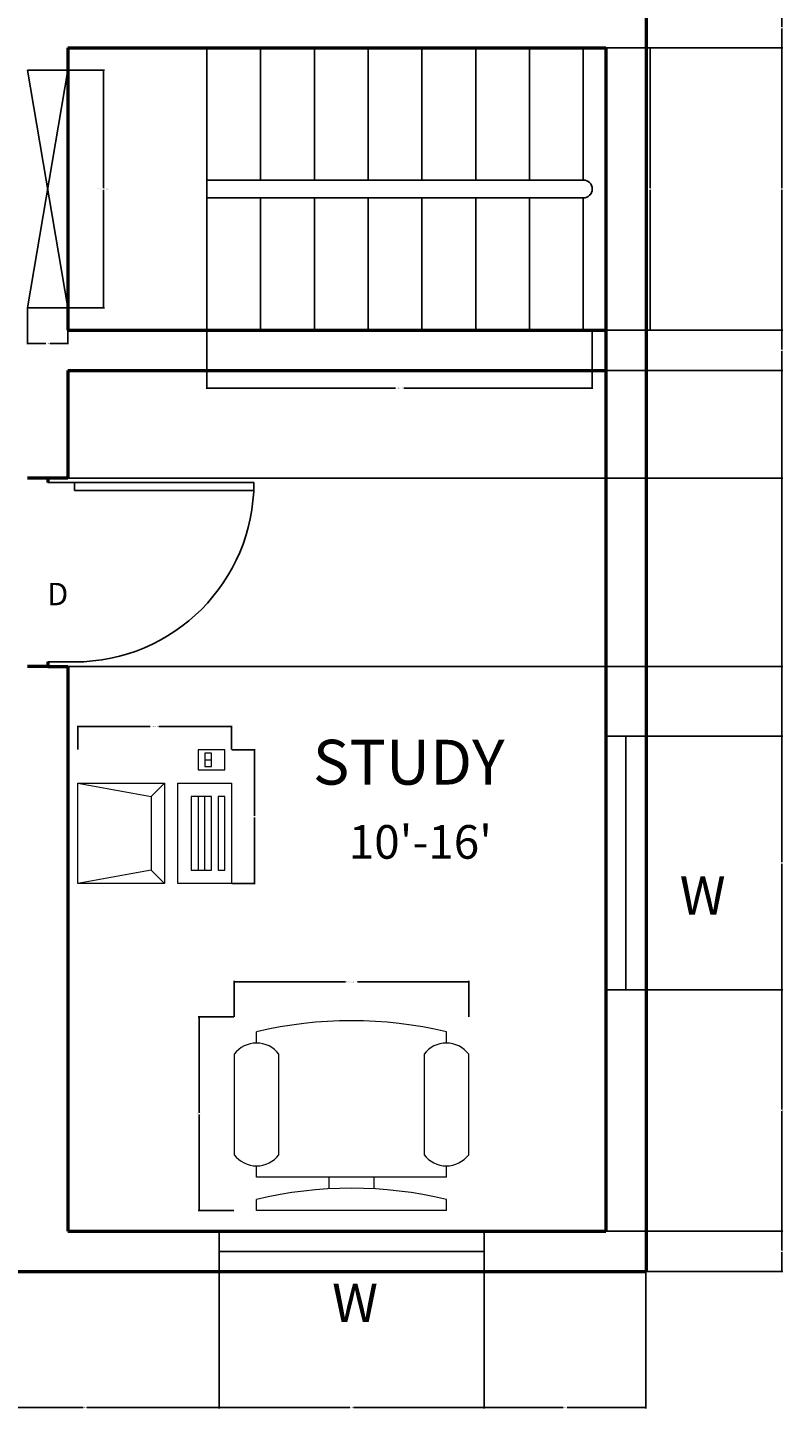
# Model space of a CAD drawing. Units: inches. Extents: x 2164 to 3752, y 2015 to 2629.
# Tile 6 of 8: x 3583 to 3752, y 2015 to 2323. Entities that reach past the tile are written whole.
import ezdxf
from ezdxf.enums import TextEntityAlignment as Align

# ---------------------------------------------------------------- set-up
doc = ezdxf.new("R2010")
doc.units = ezdxf.units.IN
for name, color, linetype, lineweight in [('A-ANNO-DIMS', 2, 'Continuous', 18), ('A-ANNO-TEXT', 7, 'Continuous', 25), ('A-AREA-IDEN', 3, 'Continuous', 25), ('A-DOOR', 3, 'Continuous', 25), ('A-FLOR-STRS', 2, 'Continuous', 25), ('A-FURN', 8, 'Continuous', 18), ('A-GLAZ', 4, 'Continuous', 25), ('A-WALL', 7, 'Continuous', 50)]:
    doc.layers.add(name, color=color, linetype=linetype, lineweight=lineweight)
doc.styles.get("Standard").update_dxf_attribs({"font": 'arial.ttf'})
doc.dimstyles.get("Standard").update_dxf_attribs({"dimtxt": 0.18, "dimasz": 0.18, "dimexe": 0.18, "dimexo": 0.0625, "dimgap": 0.09, "dimtad": 0, "dimtih": 1, "dimtoh": 1, "dimdec": 4, "dimzin": 0, "dimdsep": 46, "dimtxsty": 'Standard', "dimcen": 0.09, "dimadec": 0, "dimazin": 0, "dimtfac": 1, "dimtdec": 4, "dimtofl": 0, "dimtmove": 0, "dimatfit": 3, "dimfxl": 1, "dimtolj": 1, "dimtzin": 0, "dimarcsym": 0})

# ---------------------------------------------------------------- blocks, each defined once
blk = doc.blocks.new('*U7')
for p, q in [((0, 0), (0, -6)), ((40, 0), (40, -6))]:
    blk.add_line(p, q)
blk.add_lwpolyline([(0, 0), (0, 40), (1.75, 40), (1.75, 0)], close=True)
blk.add_arc((0, 0), 40, 0, 90)
blk = doc.blocks.new('Chair - Desk')
for p, q in [((-8.5, 0), (-8.5, -1)), ((-8.5, 0), (8.5, 0)), ((8.5, 0), (8.5, -1)), ((-2, -3), (-2, -1.9355)), ((2, -1.9576), (2, -3)), ((-8.5, -3), (-8.5, -4)), ((-8.5, -3), (8.5, -3)), ((8.5, -3), (8.5, -4)), ((-10.5, -5), (-10.5, -14)), ((-6.5, -14), (-6.5, -5)), ((6.5, -5), (6.5, -14)), ((10.5, -14), (10.5, -5)), ((-8.5, -15), (-8.5, -16)), ((8.5, -15), (8.5, -16))]:
    blk.add_line(p, q)
for centre, radius, start, end in [((0, 34.625), 36.625, 256.5803, 283.4197), ((-8.5, -6.5), 2.5, 36.8699, 143.1301), ((8.5, -6.5), 2.5, 36.8699, 143.1301), ((-8.5, -12.5), 2.5, 216.8699, 323.1301), ((8.5, -12.5), 2.5, 216.8699, 323.1301), ((0, 19.625), 36.625, 256.5803, 283.4197)]:
    blk.add_arc(centre, radius, start, end)
blk = doc.blocks.new('Computer Terminal')
for p, q in [((-10, 11.5), (5, 11.5)), ((-8, 0.5), (-10, 11.5)), ((-10, -1.5), (-10, 11.5)), ((5, 11.5), (3, 0.5)), ((5, 11.5), (5, -1.5)), ((-10, -1.5), (-8, 0.5)), ((3, 0.5), (-8, 0.5)), ((3, 0.5), (5, -1.5)), ((5, -1.5), (-10, -1.5)), ((-10, -11.5), (-10, -3.5)), ((-10, -3.5), (5, -3.5)), ((5, -3.5), (5, -11.5)), ((-8, -5.5), (-8, -8.5)), ((3, -5.5), (-8, -5.5)), ((3, -8.5), (3, -5.5)), ((3, -6.5), (-8, -6.5)), ((-8, -7.5), (3, -7.5)), ((10, -6.5), (7, -6.5)), ((7, -6.5), (7, -10.5)), ((9.5, -7.5), (7.5, -7.5)), ((7.5, -7.5), (7.5, -8.5)), ((8.5, -7.5), (8.5, -8.5)), ((9.5, -8.5), (9.5, -7.5)), ((10, -10.5), (10, -6.5)), ((-8, -8.5), (3, -8.5)), ((-8, -9.5), (-8, -10.5)), ((3, -9.5), (-8, -9.5)), ((3, -10.5), (3, -9.5)), ((7.5, -8.5), (9.5, -8.5)), ((5, -11.5), (-10, -11.5)), ((-8, -10.5), (3, -10.5)), ((7, -10.5), (10, -10.5))]:
    blk.add_line(p, q)
blk = doc.blocks.new('STAIR-HANDRAIL')
for p, q in [((84, 63), (84, 33.5)), ((0, 33.5), (84, 33.5)), ((0, 29.5), (84, 29.5)), ((84, 29.5), (84, 0))]:
    blk.add_line(p, q)
blk.add_arc((84, 31.5), 2, 270, 90)
blk = doc.blocks.new('VENT-OPENING')
for p, q in [((9, 53), (0, 53)), ((9, 53), (0, 0)), ((9, 0), (0, 53)), ((9, 0), (0, 0))]:
    blk.add_line(p, q)
blk = doc.blocks.new('*D25')
at = {"layer": 'A-ANNO-DIMS', "color": 0, "lineweight": -2, "transparency": 16777216}
for p, q in [((3629.5, 2102.57), (3629.5, 2110.54)), ((3629.68, 2110.36), (3654.34, 2110.36)), ((3681.65, 2110.36), (3656.99, 2110.36)), ((3681.83, 2102.57), (3681.83, 2110.54))]:
    blk.add_line(p, q, dxfattribs=at)
at = {"layer": 'A-ANNO-DIMS', "color": 0, "transparency": 16777216}
for points in [[(3629.68, 2110.39), (3629.68, 2110.33), (3629.5, 2110.36)], [(3681.65, 2110.39), (3681.65, 2110.33), (3681.83, 2110.36)]]:
    blk.add_solid(points, dxfattribs=at)
at = {"layer": 'Defpoints', "color": 0, "transparency": 16777216}
for p in [(3629.5, 2110.36), (3629.5, 2102.51), (3681.83, 2102.51)]:
    blk.add_point(p, dxfattribs=at)
at = {"layer": 'A-ANNO-DIMS', "color": 0, "transparency": 16777216, "insert": (3655.66, 2110.36), "char_height": 0.18, "attachment_point": 5}
blk.add_mtext('\\A1;DESK CHAIR 52 TYP.', dxfattribs=at)
blk = doc.blocks.new('*D26')
at = {"layer": 'A-ANNO-DIMS', "color": 0, "lineweight": -2, "transparency": 16777216}
for p, q in [((3629.44, 2102.51), (3621.47, 2102.51)), ((3621.65, 2102.33), (3621.65, 2081.1)), ((3621.65, 2059.5), (3621.65, 2080.73)), ((3629.44, 2059.32), (3621.47, 2059.32))]:
    blk.add_line(p, q, dxfattribs=at)
at = {"layer": 'A-ANNO-DIMS', "color": 0, "transparency": 16777216}
for points in [[(3621.62, 2102.33), (3621.68, 2102.33), (3621.65, 2102.51)], [(3621.62, 2059.5), (3621.68, 2059.5), (3621.65, 2059.32)]]:
    blk.add_solid(points, dxfattribs=at)
at = {"layer": 'Defpoints', "color": 0, "transparency": 16777216}
for p in [(3629.5, 2102.51), (3621.65, 2059.32), (3629.5, 2059.32)]:
    blk.add_point(p, dxfattribs=at)
at = {"layer": 'A-ANNO-DIMS', "color": 0, "transparency": 16777216, "insert": (3621.65, 2080.92), "char_height": 0.18, "attachment_point": 5}
blk.add_mtext('\\A1;43 TYP.', dxfattribs=at)
blk = doc.blocks.new('*D31')
at = {"layer": 'A-ANNO-DIMS', "color": 0, "lineweight": -2, "transparency": 16777216}
for p, q in [((3623.39, 2255.65), (3623.39, 2242.64)), ((3709.39, 2255.65), (3709.39, 2242.64)), ((3623.57, 2242.82), (3665.46, 2242.82)), ((3709.21, 2242.82), (3667.33, 2242.82))]:
    blk.add_line(p, q, dxfattribs=at)
at = {"layer": 'A-ANNO-DIMS', "color": 0, "transparency": 16777216}
for points in [[(3623.57, 2242.85), (3623.57, 2242.79), (3623.39, 2242.82)], [(3709.21, 2242.85), (3709.21, 2242.79), (3709.39, 2242.82)]]:
    blk.add_solid(points, dxfattribs=at)
at = {"layer": 'Defpoints', "color": 0, "transparency": 16777216}
for p in [(3623.39, 2255.72), (3709.39, 2255.72), (3709.39, 2242.82)]:
    blk.add_point(p, dxfattribs=at)
at = {"layer": 'A-ANNO-DIMS', "color": 0, "transparency": 16777216, "insert": (3666.39, 2242.82), "char_height": 0.18, "attachment_point": 5}
blk.add_mtext('\\A1;STAIR 86 TYP.', dxfattribs=at)
blk = doc.blocks.new('*D32')
at = {"layer": 'A-ANNO-DIMS', "color": 0, "lineweight": -2, "transparency": 16777216}
for p, q in [((3709.46, 2318.72), (3722.47, 2318.72)), ((3722.29, 2318.54), (3722.29, 2287.4)), ((3722.29, 2255.9), (3722.29, 2287.04)), ((3709.46, 2255.72), (3722.47, 2255.72))]:
    blk.add_line(p, q, dxfattribs=at)
at = {"layer": 'A-ANNO-DIMS', "color": 0, "transparency": 16777216}
for points in [[(3722.26, 2318.54), (3722.32, 2318.54), (3722.29, 2318.72)], [(3722.26, 2255.9), (3722.32, 2255.9), (3722.29, 2255.72)]]:
    blk.add_solid(points, dxfattribs=at)
at = {"layer": 'Defpoints', "color": 0, "transparency": 16777216}
for p in [(3709.39, 2318.72), (3722.29, 2318.72), (3709.39, 2255.72)]:
    blk.add_point(p, dxfattribs=at)
at = {"layer": 'A-ANNO-DIMS', "color": 0, "transparency": 16777216, "insert": (3722.29, 2287.22), "char_height": 0.18, "attachment_point": 5}
blk.add_mtext('\\A1;63 TYP.', dxfattribs=at)
blk = doc.blocks.new('*D33')
at = {"layer": 'A-ANNO-DIMS', "color": 0, "lineweight": -2, "transparency": 16777216}
for p, q in [((3592.46, 2313.72), (3600.52, 2313.72)), ((3600.34, 2313.54), (3600.34, 2287.4)), ((3600.34, 2260.9), (3600.34, 2287.03)), ((3592.46, 2260.72), (3600.52, 2260.72))]:
    blk.add_line(p, q, dxfattribs=at)
at = {"layer": 'A-ANNO-DIMS', "color": 0, "transparency": 16777216}
for points in [[(3600.31, 2313.54), (3600.37, 2313.54), (3600.34, 2313.72)], [(3600.31, 2260.9), (3600.37, 2260.9), (3600.34, 2260.72)]]:
    blk.add_solid(points, dxfattribs=at)
at = {"layer": 'Defpoints', "color": 0, "transparency": 16777216}
for p in [(3592.39, 2313.72), (3600.34, 2313.72), (3592.39, 2260.72)]:
    blk.add_point(p, dxfattribs=at)
at = {"layer": 'A-ANNO-DIMS', "color": 0, "transparency": 16777216, "insert": (3600.34, 2287.22), "char_height": 0.18, "attachment_point": 5}
blk.add_mtext('\\A1;VENT OPENING 53 TYP.', dxfattribs=at)
blk = doc.blocks.new('*D34')
at = {"layer": 'A-ANNO-DIMS', "color": 0, "lineweight": -2, "transparency": 16777216}
for p, q in [((3583.39, 2260.65), (3583.39, 2252.59)), ((3592.39, 2260.65), (3592.39, 2252.59)), ((3583.57, 2252.77), (3587.44, 2252.77)), ((3592.21, 2252.77), (3588.35, 2252.77))]:
    blk.add_line(p, q, dxfattribs=at)
at = {"layer": 'A-ANNO-DIMS', "color": 0, "transparency": 16777216}
for points in [[(3583.57, 2252.8), (3583.57, 2252.74), (3583.39, 2252.77)], [(3592.21, 2252.8), (3592.21, 2252.74), (3592.39, 2252.77)]]:
    blk.add_solid(points, dxfattribs=at)
at = {"layer": 'Defpoints', "color": 0, "transparency": 16777216}
for p in [(3583.39, 2260.72), (3592.39, 2260.72), (3592.39, 2252.77)]:
    blk.add_point(p, dxfattribs=at)
at = {"layer": 'A-ANNO-DIMS', "color": 0, "transparency": 16777216, "insert": (3587.89, 2252.77), "char_height": 0.18, "attachment_point": 5}
blk.add_mtext('\\A1;9 TYP.', dxfattribs=at)
blk = doc.blocks.new('*D45')
at = {"layer": 'A-ANNO-DIMS', "color": 0, "lineweight": -2, "transparency": 16777216}
for p, q in [((3594.57, 2162.19), (3594.57, 2167.45)), ((3594.75, 2167.27), (3610.75, 2167.27)), ((3628.7, 2167.27), (3612.7, 2167.27)), ((3628.88, 2162.19), (3628.88, 2167.45))]:
    blk.add_line(p, q, dxfattribs=at)
at = {"layer": 'A-ANNO-DIMS', "color": 0, "transparency": 16777216}
for points in [[(3594.75, 2167.3), (3594.75, 2167.24), (3594.57, 2167.27)], [(3628.7, 2167.3), (3628.7, 2167.24), (3628.88, 2167.27)]]:
    blk.add_solid(points, dxfattribs=at)
at = {"layer": 'Defpoints', "color": 0, "transparency": 16777216}
for p in [(3594.57, 2167.27), (3594.57, 2162.13), (3628.88, 2162.13)]:
    blk.add_point(p, dxfattribs=at)
at = {"layer": 'A-ANNO-DIMS', "color": 0, "transparency": 16777216, "insert": (3611.73, 2167.27), "char_height": 0.18, "attachment_point": 5}
blk.add_mtext('\\A1;COMPUTER 34', dxfattribs=at)
blk = doc.blocks.new('*D46')
at = {"layer": 'A-ANNO-DIMS', "color": 0, "lineweight": -2, "transparency": 16777216}
for p, q in [((3628.94, 2162.13), (3634.2, 2162.13)), ((3634.02, 2161.95), (3634.02, 2147.39)), ((3634.02, 2132.48), (3634.02, 2147.03)), ((3628.94, 2132.3), (3634.2, 2132.3))]:
    blk.add_line(p, q, dxfattribs=at)
at = {"layer": 'A-ANNO-DIMS', "color": 0, "transparency": 16777216}
for points in [[(3633.99, 2161.95), (3634.05, 2161.95), (3634.02, 2162.13)], [(3633.99, 2132.48), (3634.05, 2132.48), (3634.02, 2132.3)]]:
    blk.add_solid(points, dxfattribs=at)
at = {"layer": 'Defpoints', "color": 0, "transparency": 16777216}
for p in [(3628.88, 2162.13), (3634.02, 2162.13), (3628.88, 2132.3)]:
    blk.add_point(p, dxfattribs=at)
at = {"layer": 'A-ANNO-DIMS', "color": 0, "transparency": 16777216, "insert": (3634.02, 2147.21), "char_height": 0.18, "attachment_point": 5}
blk.add_mtext('\\A1;30', dxfattribs=at)
blk = doc.blocks.new('*D117')
at = {"layer": 'A-ANNO-DIMS', "color": 0, "lineweight": -2, "transparency": 16777216}
for p, q in [((3566.34, 2045.65), (3566.34, 2015.19)), ((3626.11, 2045.65), (3626.11, 2015.19)), ((3566.52, 2015.37), (3595.83, 2015.37)), ((3625.93, 2015.37), (3596.62, 2015.37))]:
    blk.add_line(p, q, dxfattribs=at)
at = {"layer": 'A-ANNO-DIMS', "color": 0, "transparency": 16777216}
for points in [[(3566.52, 2015.4), (3566.52, 2015.34), (3566.34, 2015.37)], [(3625.93, 2015.4), (3625.93, 2015.34), (3626.11, 2015.37)]]:
    blk.add_solid(points, dxfattribs=at)
at = {"layer": 'Defpoints', "color": 0, "transparency": 16777216}
for p in [(3566.34, 2045.72), (3626.11, 2045.72), (3626.11, 2015.37)]:
    blk.add_point(p, dxfattribs=at)
at = {"layer": 'A-ANNO-DIMS', "color": 0, "transparency": 16777216, "insert": (3596.23, 2015.37), "char_height": 0.18, "attachment_point": 5}
blk.add_mtext('\\A1;59.77', dxfattribs=at)
blk = doc.blocks.new('*D118')
at = {"layer": 'A-ANNO-DIMS', "color": 0, "lineweight": -2, "transparency": 16777216}
for p, q in [((3626.11, 2045.65), (3626.11, 2015.19)), ((3685.3, 2045.65), (3685.3, 2015.19)), ((3626.29, 2015.37), (3655.31, 2015.37)), ((3685.12, 2015.37), (3656.1, 2015.37))]:
    blk.add_line(p, q, dxfattribs=at)
at = {"layer": 'A-ANNO-DIMS', "color": 0, "transparency": 16777216}
for points in [[(3626.29, 2015.4), (3626.29, 2015.34), (3626.11, 2015.37)], [(3685.12, 2015.4), (3685.12, 2015.34), (3685.3, 2015.37)]]:
    blk.add_solid(points, dxfattribs=at)
at = {"layer": 'Defpoints', "color": 0, "transparency": 16777216}
for p in [(3626.11, 2045.72), (3685.3, 2045.72), (3685.3, 2015.37)]:
    blk.add_point(p, dxfattribs=at)
at = {"layer": 'A-ANNO-DIMS', "color": 0, "transparency": 16777216, "insert": (3655.71, 2015.37), "char_height": 0.18, "attachment_point": 5}
blk.add_mtext('\\A1;59.19', dxfattribs=at)
blk = doc.blocks.new('*D119')
at = {"layer": 'A-ANNO-DIMS', "color": 0, "lineweight": -2, "transparency": 16777216}
for p, q in [((3685.3, 2045.65), (3685.3, 2015.19)), ((3721.39, 2045.65), (3721.39, 2015.19)), ((3685.48, 2015.37), (3702.88, 2015.37)), ((3721.21, 2015.37), (3703.81, 2015.37))]:
    blk.add_line(p, q, dxfattribs=at)
at = {"layer": 'A-ANNO-DIMS', "color": 0, "transparency": 16777216}
for points in [[(3685.48, 2015.4), (3685.48, 2015.34), (3685.3, 2015.37)], [(3721.21, 2015.4), (3721.21, 2015.34), (3721.39, 2015.37)]]:
    blk.add_solid(points, dxfattribs=at)
at = {"layer": 'Defpoints', "color": 0, "transparency": 16777216}
for p in [(3685.3, 2045.72), (3721.39, 2045.72), (3721.39, 2015.37)]:
    blk.add_point(p, dxfattribs=at)
at = {"layer": 'A-ANNO-DIMS', "color": 0, "transparency": 16777216, "insert": (3703.35, 2015.37), "char_height": 0.18, "attachment_point": 5}
blk.add_mtext('\\A1;36.096', dxfattribs=at)
blk = doc.blocks.new('*D128')
at = {"layer": 'A-ANNO-DIMS', "color": 0, "lineweight": -2, "transparency": 16777216}
for p, q in [((3712.46, 2054.72), (3751.92, 2054.72)), ((3751.74, 2054.54), (3751.74, 2050.4)), ((3751.74, 2045.9), (3751.74, 2050.04)), ((3721.46, 2045.72), (3751.92, 2045.72))]:
    blk.add_line(p, q, dxfattribs=at)
at = {"layer": 'A-ANNO-DIMS', "color": 0, "transparency": 16777216}
for points in [[(3751.71, 2054.54), (3751.77, 2054.54), (3751.74, 2054.72)], [(3751.71, 2045.9), (3751.77, 2045.9), (3751.74, 2045.72)]]:
    blk.add_solid(points, dxfattribs=at)
at = {"layer": 'Defpoints', "color": 0, "transparency": 16777216}
for p in [(3712.39, 2054.72), (3751.74, 2054.72), (3721.39, 2045.72)]:
    blk.add_point(p, dxfattribs=at)
at = {"layer": 'A-ANNO-DIMS', "color": 0, "transparency": 16777216, "insert": (3751.74, 2050.22), "char_height": 0.18, "attachment_point": 5}
blk.add_mtext('\\A1;9', dxfattribs=at)
blk = doc.blocks.new('*D129')
at = {"layer": 'A-ANNO-DIMS', "color": 0, "lineweight": -2, "transparency": 16777216}
for p, q in [((3721.46, 2108.58), (3751.92, 2108.58)), ((3751.74, 2108.4), (3751.74, 2081.83)), ((3751.74, 2054.9), (3751.74, 2081.47)), ((3712.46, 2054.72), (3751.92, 2054.72))]:
    blk.add_line(p, q, dxfattribs=at)
at = {"layer": 'A-ANNO-DIMS', "color": 0, "transparency": 16777216}
for points in [[(3751.71, 2108.4), (3751.77, 2108.4), (3751.74, 2108.58)], [(3751.71, 2054.9), (3751.77, 2054.9), (3751.74, 2054.72)]]:
    blk.add_solid(points, dxfattribs=at)
at = {"layer": 'Defpoints', "color": 0, "transparency": 16777216}
for p in [(3721.39, 2108.58), (3751.74, 2108.58), (3712.39, 2054.72)]:
    blk.add_point(p, dxfattribs=at)
at = {"layer": 'A-ANNO-DIMS', "color": 0, "transparency": 16777216, "insert": (3751.74, 2081.65), "char_height": 0.18, "attachment_point": 5}
blk.add_mtext('\\A1;53.86', dxfattribs=at)
blk = doc.blocks.new('*D130')
at = {"layer": 'A-ANNO-DIMS', "color": 0, "lineweight": -2, "transparency": 16777216}
for p, q in [((3721.46, 2165.13), (3751.92, 2165.13)), ((3751.74, 2164.95), (3751.74, 2137.03)), ((3751.74, 2108.76), (3751.74, 2136.67)), ((3721.46, 2108.58), (3751.92, 2108.58))]:
    blk.add_line(p, q, dxfattribs=at)
at = {"layer": 'A-ANNO-DIMS', "color": 0, "transparency": 16777216}
for points in [[(3751.71, 2164.95), (3751.77, 2164.95), (3751.74, 2165.13)], [(3751.71, 2108.76), (3751.77, 2108.76), (3751.74, 2108.58)]]:
    blk.add_solid(points, dxfattribs=at)
at = {"layer": 'Defpoints', "color": 0, "transparency": 16777216}
for p in [(3721.39, 2165.13), (3751.74, 2165.13), (3721.39, 2108.58)]:
    blk.add_point(p, dxfattribs=at)
at = {"layer": 'A-ANNO-DIMS', "color": 0, "transparency": 16777216, "insert": (3751.74, 2136.85), "char_height": 0.18, "attachment_point": 5}
blk.add_mtext('\\A1;56.55', dxfattribs=at)
blk = doc.blocks.new('*D131')
at = {"layer": 'A-ANNO-DIMS', "color": 0, "lineweight": -2, "transparency": 16777216}
for p, q in [((3712.46, 2246.72), (3751.92, 2246.72)), ((3751.74, 2246.54), (3751.74, 2206.1)), ((3751.74, 2165.31), (3751.74, 2205.74)), ((3721.46, 2165.13), (3751.92, 2165.13))]:
    blk.add_line(p, q, dxfattribs=at)
at = {"layer": 'A-ANNO-DIMS', "color": 0, "transparency": 16777216}
for points in [[(3751.71, 2246.54), (3751.77, 2246.54), (3751.74, 2246.72)], [(3751.71, 2165.31), (3751.77, 2165.31), (3751.74, 2165.13)]]:
    blk.add_solid(points, dxfattribs=at)
at = {"layer": 'Defpoints', "color": 0, "transparency": 16777216}
for p in [(3712.39, 2246.72), (3751.74, 2246.72), (3721.39, 2165.13)]:
    blk.add_point(p, dxfattribs=at)
at = {"layer": 'A-ANNO-DIMS', "color": 0, "transparency": 16777216, "insert": (3751.74, 2205.92), "char_height": 0.18, "attachment_point": 5}
blk.add_mtext('\\A1;81.59', dxfattribs=at)
blk = doc.blocks.new('*D132')
at = {"layer": 'A-ANNO-DIMS', "color": 0, "lineweight": -2, "transparency": 16777216}
for p, q in [((3712.46, 2255.72), (3751.92, 2255.72)), ((3751.74, 2255.54), (3751.74, 2251.4)), ((3751.74, 2246.9), (3751.74, 2251.04)), ((3712.46, 2246.72), (3751.92, 2246.72))]:
    blk.add_line(p, q, dxfattribs=at)
at = {"layer": 'A-ANNO-DIMS', "color": 0, "transparency": 16777216}
for points in [[(3751.71, 2255.54), (3751.77, 2255.54), (3751.74, 2255.72)], [(3751.71, 2246.9), (3751.77, 2246.9), (3751.74, 2246.72)]]:
    blk.add_solid(points, dxfattribs=at)
at = {"layer": 'Defpoints', "color": 0, "transparency": 16777216}
for p in [(3712.39, 2255.72), (3751.74, 2255.72), (3712.39, 2246.72)]:
    blk.add_point(p, dxfattribs=at)
at = {"layer": 'A-ANNO-DIMS', "color": 0, "transparency": 16777216, "insert": (3751.74, 2251.22), "char_height": 0.18, "attachment_point": 5}
blk.add_mtext('\\A1;9', dxfattribs=at)
blk = doc.blocks.new('*D133')
at = {"layer": 'A-ANNO-DIMS', "color": 0, "lineweight": -2, "transparency": 16777216}
for p, q in [((3712.46, 2318.72), (3751.92, 2318.72)), ((3751.74, 2318.54), (3751.74, 2287.4)), ((3751.74, 2255.9), (3751.74, 2287.04)), ((3712.46, 2255.72), (3751.92, 2255.72))]:
    blk.add_line(p, q, dxfattribs=at)
at = {"layer": 'A-ANNO-DIMS', "color": 0, "transparency": 16777216}
for points in [[(3751.71, 2318.54), (3751.77, 2318.54), (3751.74, 2318.72)], [(3751.71, 2255.9), (3751.77, 2255.9), (3751.74, 2255.72)]]:
    blk.add_solid(points, dxfattribs=at)
at = {"layer": 'Defpoints', "color": 0, "transparency": 16777216}
for p in [(3712.39, 2318.72), (3751.74, 2318.72), (3712.39, 2255.72)]:
    blk.add_point(p, dxfattribs=at)
at = {"layer": 'A-ANNO-DIMS', "color": 0, "transparency": 16777216, "insert": (3751.74, 2287.22), "char_height": 0.18, "attachment_point": 5}
blk.add_mtext('\\A1;63', dxfattribs=at)
blk = doc.blocks.new('*D134')
at = {"layer": 'A-ANNO-DIMS', "color": 0, "lineweight": -2, "transparency": 16777216}
for p, q in [((3712.46, 2327.72), (3751.92, 2327.72)), ((3751.74, 2327.54), (3751.74, 2323.4)), ((3751.74, 2318.9), (3751.74, 2323.04)), ((3712.46, 2318.72), (3751.92, 2318.72))]:
    blk.add_line(p, q, dxfattribs=at)
at = {"layer": 'A-ANNO-DIMS', "color": 0, "transparency": 16777216}
for points in [[(3751.71, 2327.54), (3751.77, 2327.54), (3751.74, 2327.72)], [(3751.71, 2318.9), (3751.77, 2318.9), (3751.74, 2318.72)]]:
    blk.add_solid(points, dxfattribs=at)
at = {"layer": 'Defpoints', "color": 0, "transparency": 16777216}
for p in [(3712.39, 2327.72), (3751.74, 2327.72), (3712.39, 2318.72)]:
    blk.add_point(p, dxfattribs=at)
at = {"layer": 'A-ANNO-DIMS', "color": 0, "transparency": 16777216, "insert": (3751.74, 2323.22), "char_height": 0.18, "attachment_point": 5}
blk.add_mtext('\\A1;9', dxfattribs=at)
blk = doc.blocks.new('*D148')
at = {"layer": 'A-ANNO-DIMS', "color": 0, "lineweight": -2, "transparency": 16777216}
for p, q in [((3583.46, 2222.72), (3751.92, 2222.72)), ((3751.74, 2222.54), (3751.74, 2201.9)), ((3751.74, 2180.9), (3751.74, 2201.54)), ((3583.46, 2180.72), (3751.92, 2180.72))]:
    blk.add_line(p, q, dxfattribs=at)
at = {"layer": 'A-ANNO-DIMS', "color": 0, "transparency": 16777216}
for points in [[(3751.71, 2222.54), (3751.77, 2222.54), (3751.74, 2222.72)], [(3751.71, 2180.9), (3751.77, 2180.9), (3751.74, 2180.72)]]:
    blk.add_solid(points, dxfattribs=at)
at = {"layer": 'Defpoints', "color": 0, "transparency": 16777216}
for p in [(3583.39, 2222.72), (3751.74, 2222.72), (3583.39, 2180.72)]:
    blk.add_point(p, dxfattribs=at)
at = {"layer": 'A-ANNO-DIMS', "color": 0, "transparency": 16777216, "insert": (3751.74, 2201.72), "char_height": 0.18, "attachment_point": 5}
blk.add_mtext('\\A1;42', dxfattribs=at)

msp = doc.modelspace()

# ---------------------------------------------------------------- linework, layer by layer
at = {"layer": 'A-FLOR-STRS'}
for p, q in [((3623.395, 2318.7172), (3623.395, 2255.7172)), ((3635.395, 2318.7172), (3635.395, 2289.2172)), ((3647.395, 2318.7172), (3647.395, 2289.2172)), ((3659.395, 2318.7172), (3659.395, 2289.2172)), ((3671.395, 2318.7172), (3671.395, 2289.2172)), ((3683.395, 2318.7172), (3683.395, 2289.2172)), ((3695.395, 2318.7172), (3695.395, 2289.2172)), ((3635.395, 2285.2172), (3635.395, 2255.7172)), ((3647.395, 2285.2172), (3647.395, 2255.7172)), ((3659.395, 2285.2172), (3659.395, 2255.7172)), ((3671.395, 2285.2172), (3671.395, 2255.7172)), ((3683.395, 2285.2172), (3683.395, 2255.7172)), ((3695.395, 2285.2172), (3695.395, 2255.7172))]:
    msp.add_line(p, q, dxfattribs=at)
at = {"layer": 'A-GLAZ'}
for p, q in [((3712.395, 2165.1259), (3721.395, 2165.1259)), ((3716.895, 2108.5768), (3716.895, 2165.1259)), ((3712.395, 2108.5768), (3721.395, 2108.5768)), ((3626.1138, 2054.7172), (3626.1138, 2045.7172)), ((3685.2989, 2054.7172), (3685.2989, 2045.7172)), ((3685.2989, 2050.2172), (3626.1138, 2050.2172))]:
    msp.add_line(p, q, dxfattribs=at)
at = {"layer": 'A-WALL'}
for p, q in [((3721.395, 2528.7172), (3721.395, 2045.7172)), ((3592.395, 2318.7172), (3592.395, 2255.7172)), ((3592.395, 2318.7172), (3712.395, 2318.7172)), ((3712.395, 2318.7172), (3712.395, 2054.7172)), ((3592.395, 2255.7172), (3712.395, 2255.7172)), ((3592.395, 2246.7172), (3712.395, 2246.7172)), ((3592.395, 2246.7172), (3592.395, 2222.7172)), ((3592.395, 2222.7172), (3583.395, 2222.7172)), ((3587.895, 2222.7172), (3587.895, 2221.7172)), ((3587.895, 2181.7172), (3587.895, 2180.7172)), ((3587.895, 2180.7172), (3583.395, 2180.7172)), ((3587.895, 2180.7172), (3592.395, 2180.7172)), ((3592.395, 2180.7172), (3592.395, 2054.7172)), ((3592.395, 2054.7172), (3712.395, 2054.7172)), ((3400.395, 2045.7172), (3721.395, 2045.7172))]:
    msp.add_line(p, q, dxfattribs=at)

# ---------------------------------------------------------------- block references
at = {"layer": 'A-DOOR', "rotation": 270}
msp.add_blockref('*U7', (3593.895, 2221.7172), dxfattribs=at)
at = {"layer": 'A-FLOR-STRS'}
msp.add_blockref('STAIR-HANDRAIL', (3623.395, 2255.717), dxfattribs=at)
at = {"layer": 'A-FURN'}
for name, p, xscale, yscale, zscale, rotation in [('Computer Terminal', (3611.7252, 2147.2108), 1.491520429784396, 1.491520429784396, 1.491520429784396, 90), ('Chair - Desk', (3655.6628, 2059.3209), 2.491772613573976, 2.491772613573976, 2.491772613573976, 180)]:
    msp.add_blockref(name, p, dxfattribs=dict(at, xscale=xscale, yscale=yscale, zscale=zscale, rotation=rotation))
at = {"layer": 'A-GLAZ'}
msp.add_blockref('VENT-OPENING', (3583.395, 2260.717), dxfattribs=at)

# ---------------------------------------------------------------- texts
at = {"layer": 'A-ANNO-TEXT'}
msp.add_text('D', height=5, dxfattribs=at).set_placement((3587.7796, 2194.353))
for p in [(3734.0354, 2128.4875), (3656.4672, 2037.6204)]:
    msp.add_text('W', height=8.5558, dxfattribs=at).set_placement(p, align=Align.MIDDLE)
at = {"layer": 'A-AREA-IDEN'}
for s, height, p in [('STUDY', 10, (3647.0594, 2154.3419)), ("10'-16'", 7.5, (3655.064, 2137.8119))]:
    msp.add_text(s, height=height, dxfattribs=at).set_placement(p)

# ---------------------------------------------------------------- dimensions: what is measured, and where the dimension line sits
at = {"layer": 'A-ANNO-DIMS'}
for base, p1, p2, override, picture, middle in [((3751.745, 2327.7172), (3712.395, 2318.7172), (3712.395, 2327.7172), {"dimdec": 0, "dimlfac": 1, "dimrnd": 0, "dimzin": 0, "dimdsep": 46, "dimlunit": 2}, '*D134', (3751.745, 2323.2172)), ((3751.745, 2318.7172), (3712.395, 2255.7172), (3712.395, 2318.7172), {"dimdec": 0, "dimlfac": 1, "dimrnd": 0, "dimzin": 0, "dimdsep": 46, "dimlunit": 2}, '*D133', (3751.745, 2287.2172)), ((3751.745, 2255.7172), (3712.395, 2246.7172), (3712.395, 2255.7172), {"dimdec": 0, "dimlfac": 1, "dimrnd": 0, "dimzin": 0, "dimdsep": 46, "dimlunit": 2}, '*D132', (3751.745, 2251.2172)), ((3751.745, 2246.7172), (3721.395, 2165.1259), (3712.395, 2246.7172), {"dimdec": 2, "dimlfac": 1, "dimrnd": 0, "dimzin": 0, "dimdsep": 46, "dimlunit": 2}, '*D131', (3751.745, 2205.9216)), ((3751.745, 2222.7172), (3583.395, 2180.7172), (3583.395, 2222.7172), {"dimdec": 0, "dimlfac": 1, "dimrnd": 0, "dimzin": 0, "dimdsep": 46, "dimlunit": 2}, '*D148', (3751.745, 2201.7172)), ((3751.745, 2165.1259), (3721.395, 2108.5768), (3721.395, 2165.1259), {"dimdec": 2, "dimlfac": 1, "dimrnd": 0, "dimzin": 0, "dimdsep": 46, "dimlunit": 2}, '*D130', (3751.745, 2136.8514)), ((3634.0234, 2162.126), (3628.8777, 2132.2956), (3628.8777, 2162.126), {"dimdec": 0, "dimrnd": 0, "dimzin": 0, "dimlunit": 2}, '*D46', (3634.0234, 2147.2108)), ((3751.745, 2108.5768), (3712.395, 2054.7172), (3721.395, 2108.5768), {"dimdec": 2, "dimlfac": 1, "dimrnd": 0, "dimzin": 0, "dimdsep": 46, "dimlunit": 2}, '*D129', (3751.745, 2081.647)), ((3751.745, 2054.7172), (3721.395, 2045.7172), (3712.395, 2054.7172), {"dimdec": 0, "dimlfac": 1, "dimrnd": 0, "dimzin": 0, "dimdsep": 46, "dimlunit": 2}, '*D128', (3751.745, 2050.2172))]:
    dim = msp.add_linear_dim(base=base, p1=p1, p2=p2, angle=90, dimstyle='Standard', override=override, dxfattribs=at)
    dim.commit()
    dim.dimension.update_dxf_attribs({"geometry": picture, "text_midpoint": middle})
for base, p1, p2, angle, text, picture, middle in [((3722.295, 2318.7172), (3709.395, 2255.7172), (3709.395, 2318.7172), 90, '<> TYP.', '*D32', (3722.295, 2287.2172)), ((3600.345, 2313.7172), (3592.395, 2260.7172), (3592.395, 2313.7172), 90, 'VENT OPENING <> TYP.', '*D33', (3600.345, 2287.2172)), ((3594.5727, 2167.2718), (3628.8777, 2162.126), (3594.5727, 2162.126), 180, 'COMPUTER <>', '*D45', (3611.7252, 2167.2718)), ((3629.4992, 2110.3607), (3681.8264, 2102.5116), (3629.4992, 2102.5116), 180, 'DESK CHAIR <> TYP.', '*D25', (3655.6628, 2110.3607)), ((3621.6501, 2059.3209), (3629.4992, 2102.5116), (3629.4992, 2059.3209), 270, '<> TYP.', '*D26', (3621.6501, 2080.9163))]:
    dim = msp.add_linear_dim(base=base, p1=p1, p2=p2, angle=angle, text=text, dimstyle='Standard', override={"dimdec": 0, "dimrnd": 0, "dimzin": 0, "dimlunit": 2}, dxfattribs=at)
    dim.commit()
    dim.dimension.update_dxf_attribs({"geometry": picture, "text_midpoint": middle})
for base, p1, p2, text, picture, middle in [((3592.395, 2252.7672), (3583.395, 2260.7172), (3592.395, 2260.7172), '<> TYP.', '*D34', (3587.895, 2252.7672)), ((3709.395, 2242.8172), (3623.395, 2255.7172), (3709.395, 2255.7172), 'STAIR <> TYP.', '*D31', (3666.395, 2242.8172))]:
    dim = msp.add_linear_dim(base=base, p1=p1, p2=p2, text=text, dimstyle='Standard', override={"dimdec": 0, "dimrnd": 0, "dimzin": 0, "dimlunit": 2}, dxfattribs=at)
    dim.commit()
    dim.dimension.update_dxf_attribs({"geometry": picture, "text_midpoint": middle})
for base, p1, p2, override, picture, middle in [((3626.1138, 2015.3672), (3566.3421, 2045.7172), (3626.1138, 2045.7172), {"dimdec": 2, "dimlfac": 1, "dimrnd": 0, "dimzin": 0, "dimdsep": 46, "dimlunit": 2}, '*D117', (3596.2279, 2015.3672)), ((3685.2989, 2015.3672), (3626.1138, 2045.7172), (3685.2989, 2045.7172), {"dimdec": 2, "dimlfac": 1, "dimrnd": 0, "dimzin": 0, "dimdsep": 46, "dimlunit": 2}, '*D118', (3655.7064, 2015.3672)), ((3721.395, 2015.3672), (3685.2989, 2045.7172), (3721.395, 2045.7172), {"dimdec": 3, "dimlfac": 1, "dimrnd": 0, "dimzin": 0, "dimdsep": 46, "dimlunit": 2}, '*D119', (3703.3469, 2015.3672))]:
    dim = msp.add_linear_dim(base=base, p1=p1, p2=p2, dimstyle='Standard', override=override, dxfattribs=at)
    dim.commit()
    dim.dimension.update_dxf_attribs({"geometry": picture, "text_midpoint": middle})

doc.saveas('drawing.dxf')
